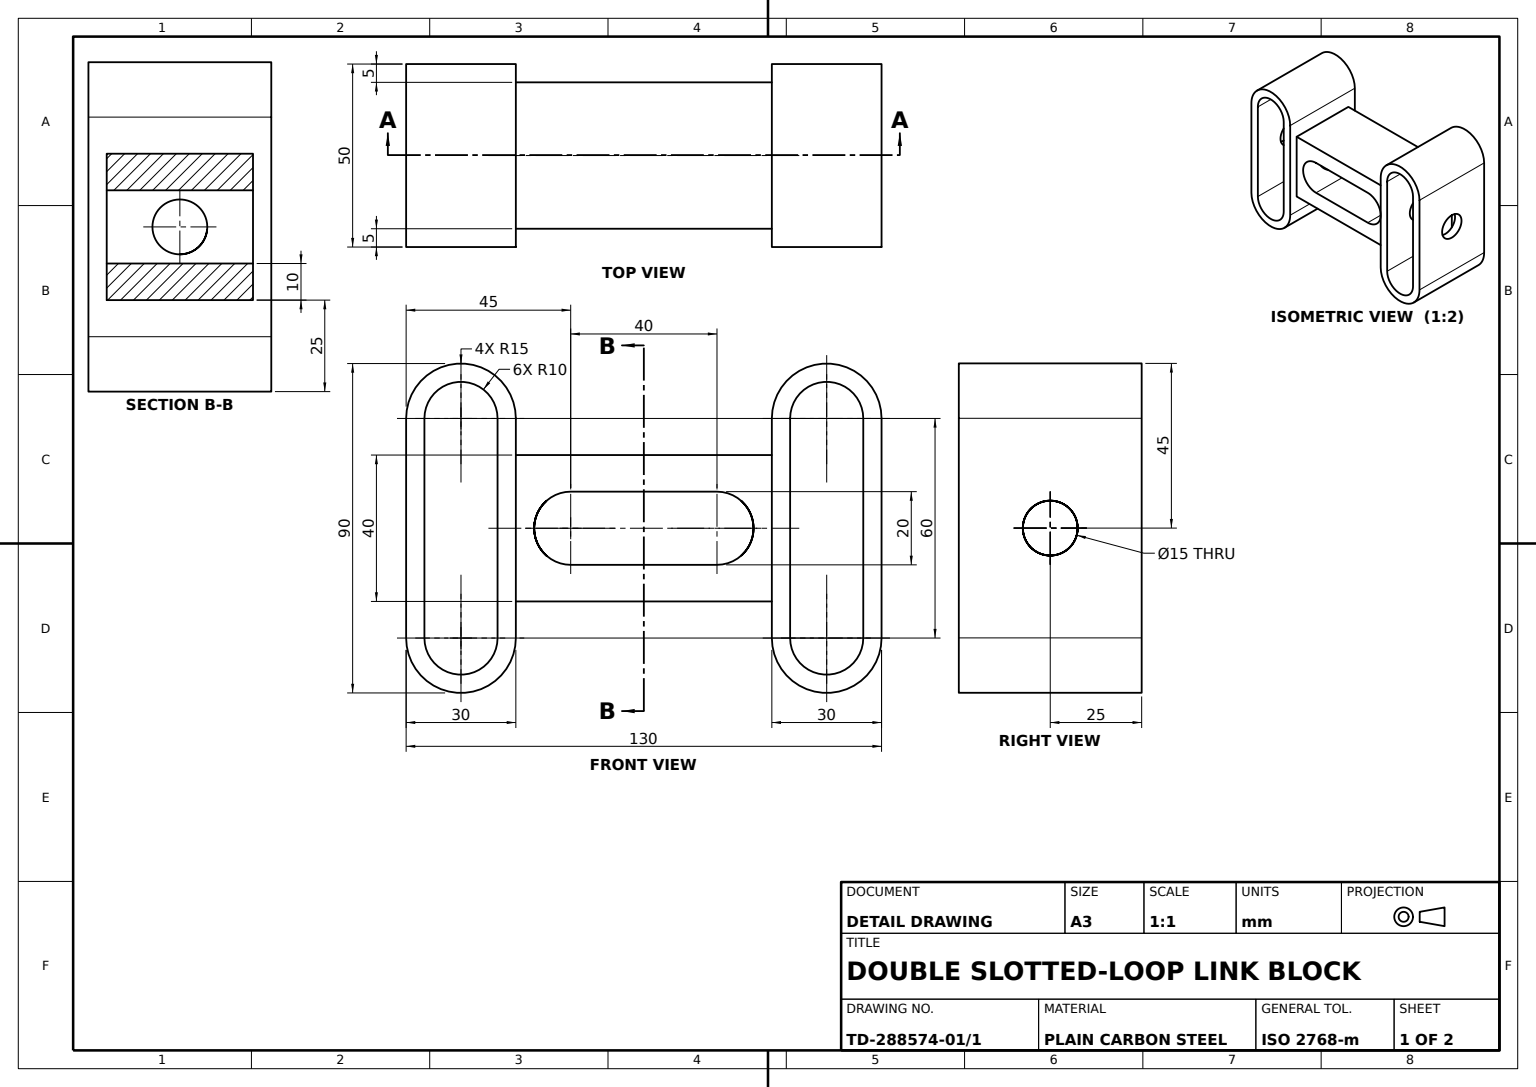
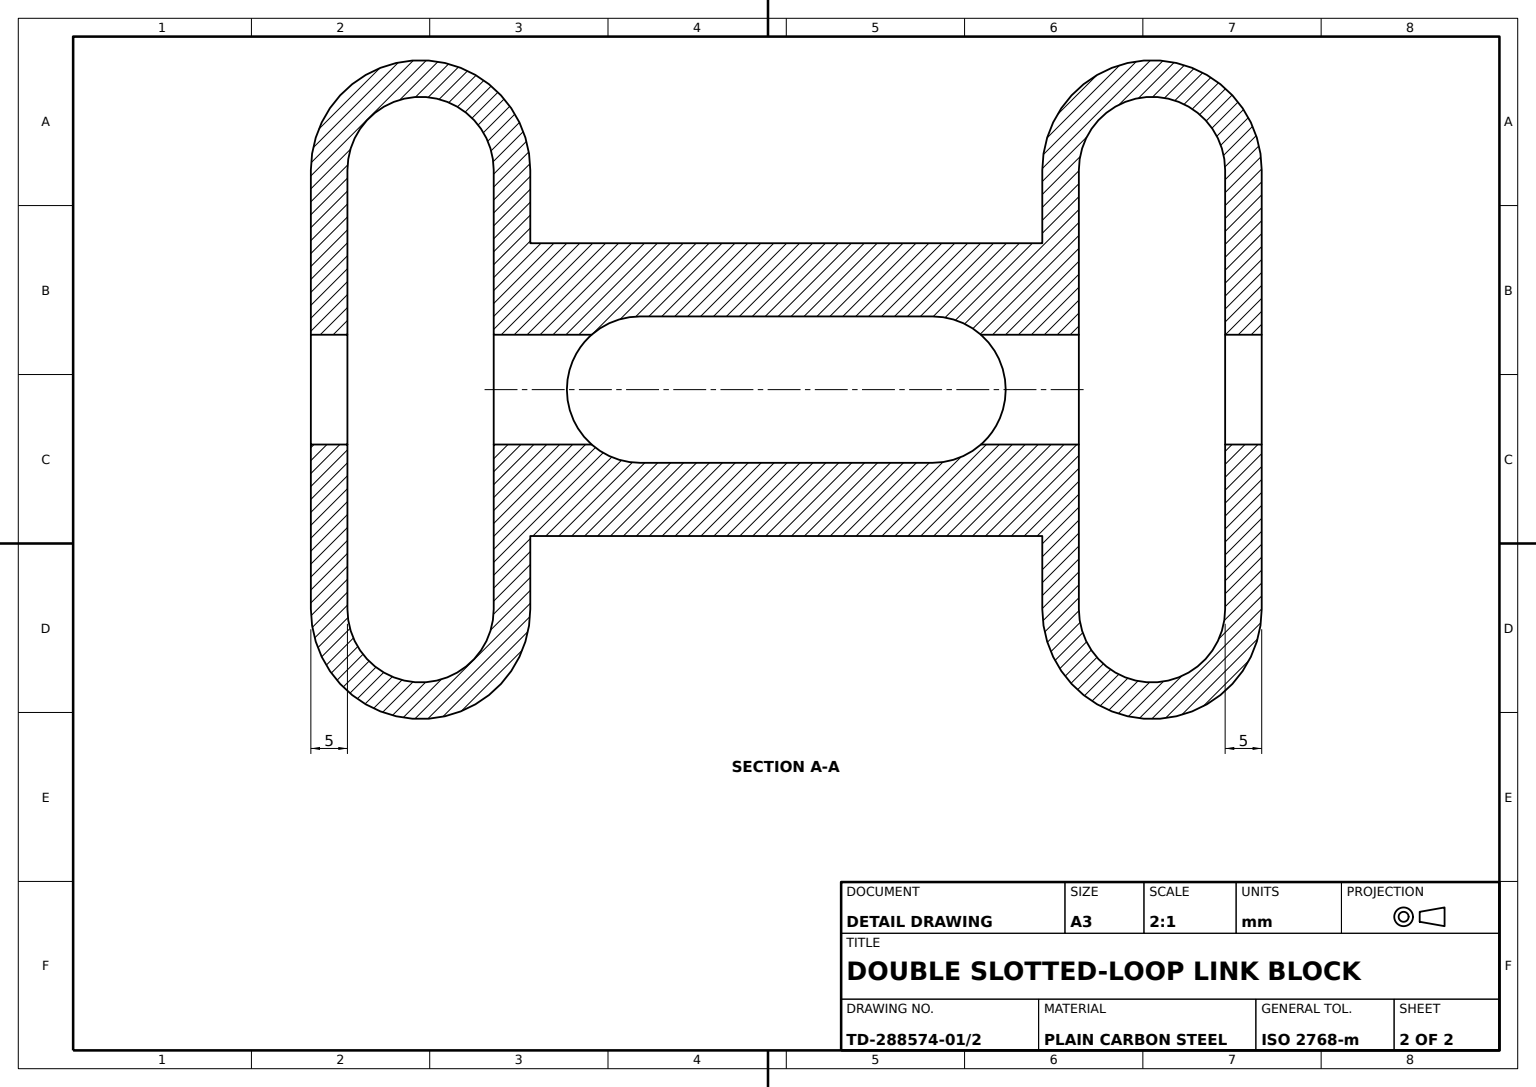
SolidWorks part; units mm, degrees
material "Plain Carbon Steel"
ref_plane "Front Plane" through (0, 0, 0) normal (0, 0, 1) x (1, 0, 0)
ref_plane "Top Plane" through (0, 0, 0) normal (0, 1, 0) x (1, 0, 0)
ref_plane "Right Plane" through (0, 0, 0) normal (1, 0, 0) x (0, 0, -1)
sketch "End Plates Profile" plane through (0, 0, 0) normal (0, 0, 1) x (1, 0, 0)
  line L0 (0, 30) -> (0, -30) construction
  line L1 (10, 30) -> (10, -30)
  line L2 (15, 30) -> (15, -30)
  line L3 (-15, 30) -> (-15, -30)
  line L4 (0, 30) -> (0, -30) construction
  line L5 (-10, 30) -> (-10, -30)
  line L6 (100, 30) -> (100, -30) construction
  line L7 (115, 30) -> (115, -30)
  line L8 (85, 30) -> (85, -30)
  line L9 (100, 30) -> (100, -30) construction
  line L10 (110, 30) -> (110, -30)
  line L11 (90, 30) -> (90, -30)
  arc A0 (15, 30) -> (-15, 30) centre (0, 30) ccw
  arc A1 (-15, -30) -> (15, -30) centre (0, -30) ccw
  arc A2 (10, 30) -> (-10, 30) centre (0, 30) ccw
  arc A3 (-10, -30) -> (10, -30) centre (0, -30) ccw
  arc A4 (115, 30) -> (85, 30) centre (100, 30) ccw
  arc A5 (85, -30) -> (115, -30) centre (100, -30) ccw
  arc A6 (110, 30) -> (90, 30) centre (100, 30) ccw
  arc A7 (90, -30) -> (110, -30) centre (100, -30) ccw
  point P3 (0, 0)
  point P5 (0, 0)
  point P15 (100, 0)
  point P22 (100, 0)
  dimension "D1" = 15
  dimension "D2" = 10
  dimension "D5" = 15
  dimension "D6" = 10
  dimension "D3" = 60
  dimension "D4" = 30
  dimension "D7" = 60
  dimension "D8" = 130
  dimension "D9" = 30
extrude "End Plates" add sketch "End Plates Profile" along normal blind 50
ref_plane "Web Mid Plane" through (0, 0, 25) normal (0, 0, 1) x (1, 0, 0)
sketch "Centre Web Profile" plane through (0, 0, 25) normal (0, 0, 1) x (1, 0, 0)
  line L0 (15, -20) -> (15, 20)
  line L1 (15, -30) -> (15, 30) construction
  line L2 (85, 30) -> (85, -30) construction
  line L3 (15, 20) -> (85, 20)
  line L4 (15, 20) -> (15, -20)
  line L5 (15, -20) -> (85, -20)
  line L6 (85, 20) -> (85, -20)
  line L7 (30, 0) -> (70, 0) construction
  line L9 (30, 10) -> (70, 10)
  line L10 (30, -10) -> (70, -10)
  arc A0 (30, 10) -> (30, -10) centre (30, 0) ccw
  arc A1 (70, -10) -> (70, 10) centre (70, 0) ccw
  point P5 (15, 0)
  point P15 (50, 0)
  dimension "D5" = 40
  dimension "D1" = 40
  dimension "D2" = 20
  dimension "D3" = 15
  dimension "D4" = 20
  dimension "D6" = 15
extrude "Centre Web" add sketch "Centre Web Profile" along normal mid plane 40 contours L6 L3 L0 L5 A1 L10 A0 L9
sketch "Cross Hole Sketch" plane through (-15, 0, 0) normal (-1, 0, 0) x (0, 0, 1)
  line L0 (0, -45) -> (50, -45) construction
  line L1 (50, 30) -> (50, -30) construction
  circle A0 centre (25, 0) radius 7.5
  dimension "D1" = 15
  dimension "D2" = 45
  dimension "D3" = 25
extrude "Cross Hole" cut sketch "Cross Hole Sketch" against normal through all
